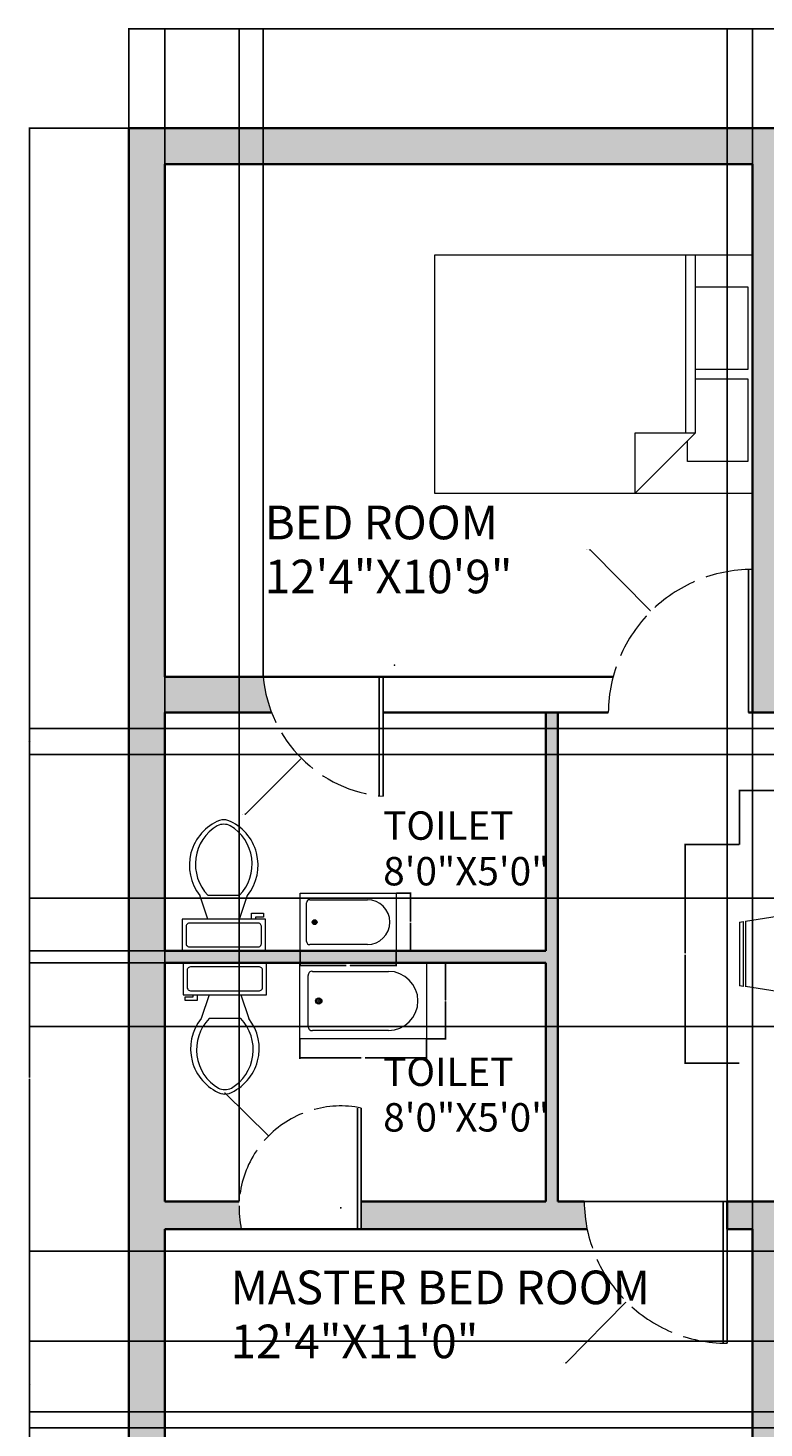
# Model space of a CAD drawing. Units: inches. Extents: x -12 to 539, y -477 to 51.
# Tile 2 of 6: x -12 to 173, y -301 to 51. Entities that reach past the tile are written whole.
import ezdxf

# ---------------------------------------------------------------- set-up
doc = ezdxf.new("R2010")
doc.units = ezdxf.units.IN
doc.header["$MEASUREMENT"] = 0
doc.linetypes.add('ACAD_ISO02W100', pattern=[15, 12, -3])
for name, color, linetype, lineweight in [('A-ANNO-DIMS', 2, 'Continuous', 18), ('A-AREA-IDEN', 7, 'Continuous', 18), ('A-DOOR', 4, 'Continuous', 25), ('A-DOOR-SWNG', 4, 'ACAD_ISO02W100', 13), ('A-FLOR-FIXT', 9, 'Continuous', 18), ('A-FURN', 8, 'Continuous', 18), ('A-WALL', 7, 'Continuous', 35)]:
    doc.layers.add(name, color=color, linetype=linetype, lineweight=lineweight)
doc.layers.add('A-WALL-PATT', color=252, linetype='Continuous', lineweight=13, true_color=0x939598)
doc.styles.get("Standard").update_dxf_attribs({"font": 'arial.ttf'})
doc.dimstyles.get("Standard").update_dxf_attribs({"dimtxt": 0.18, "dimasz": 0.18, "dimexe": 0.18, "dimexo": 0.0625, "dimgap": 0.09, "dimtad": 0, "dimtih": 1, "dimtoh": 1, "dimdec": 0, "dimzin": 0, "dimdsep": 46, "dimlunit": 3, "dimtxsty": 'Standard', "dimcen": 0.09, "dimadec": 0, "dimazin": 0, "dimtfac": 1, "dimtdec": 0, "dimtofl": 0, "dimtmove": 0, "dimatfit": 3, "dimfxl": 1, "dimtolj": 1, "dimtzin": 0, "dimarcsym": 0})

# ---------------------------------------------------------------- blocks, each defined once
blk = doc.blocks.new('Toilet - top')
for p, q in [((9.5, -6), (9.5, -2)), ((-10, -8.5), (-8, -8.5)), ((-10, -9.5), (-10, -8.5)), ((-7, -9.5), (-10, -9.5)), ((-8, -8.5), (-8, -8)), ((-7, -8), (-7, -9.5)), ((-4, -8), (-6, -14)), ((4, -8), (6, -14)), ((4, -14), (-4, -14))]:
    blk.add_line(p, q)
blk.add_lwpolyline([(10.5, -8), (10.5, 0), (-10.5, 0), (-10.5, -8)], close=True)
for points in [[(-9.5, -2), (-9.5, -6)], [(8.5, -1), (-8.5, -1)], [(-8.5, -7), (8.5, -7)]]:
    blk.add_lwpolyline(points)
for centre, radius, start, end in [((-8.62, -1.88), 0.884, 81.8699, 188.1301), ((8.62, -1.88), 0.884, 351.8699, 98.1301), ((-8.62, -6.12), 0.884, 171.8699, 278.1301), ((8.62, -6.12), 0.884, 261.8699, 8.1301), ((3.52, -21.58), 12.17, 141.4691, 247.9714), ((4.2, -21.82), 11.33, 136.3677, 238.9468), ((-3.52, -21.58), 12.17, 292.0284, 38.5307), ((-4.2, -21.82), 11.33, 301.053, 43.6321), ((0, -27.88), 4, 245.7318, 294.2682), ((0, -29), 4, 254.8605, 285.1395)]:
    blk.add_arc(centre, radius, start, end)
blk = doc.blocks.new('Bath Tub - 26 x 60 in.')
for p, q in [((8, -18), (10, -18)), ((9, -17), (9, -19))]:
    blk.add_line(p, q)
blk.add_lwpolyline([(0, -36), (0, 0), (60, 0), (60, -36)], close=True)
for points in [[(4, -30), (4, -6)], [(6, -4), (42, -4)], [(42, -32), (6, -32)]]:
    blk.add_lwpolyline(points)
for radius in [1.5, 1]:
    blk.add_circle((9, -18), radius)
for centre, radius, start, end in [((5.75, -5.75), 1.77, 81.8699, 188.1301), ((42, -18), 14, 270, 90), ((5.75, -30.25), 1.77, 171.8699, 278.1301)]:
    blk.add_arc(centre, radius, start, end)
blk = doc.blocks.new('Bed - Queen')
for p, q in [((0, -80.00003), (0, 0)), ((0, 0), (59.99999, 0)), ((59.99999, 0), (59.99999, -80.00003)), ((7.99999, -1.2), (28.79998, -1.2)), ((7.99999, -14.4), (7.99999, -1.2)), ((28.79998, -1.2), (28.79998, -14.4)), ((31.19999, -1.2), (51.99999, -1.2)), ((31.19999, -14.4), (31.19999, -1.2)), ((51.99999, -1.2), (51.99999, -16.4)), ((0, -14.4), (44.8, -14.4)), ((44.8, -16.8), (0, -16.8)), ((59.99999, -29.6), (44.8, -14.4)), ((44.8, -14.4), (44.8, -29.6)), ((51.99999, -16.4), (46.79936, -16.4)), ((44.8, -29.6), (59.99999, -29.6)), ((59.99999, -80.00003), (0, -80.00003))]:
    blk.add_line(p, q)
blk = doc.blocks.new('Dining Set - 36 x 72 in.')
for p, q in [((-22.2343, 26.00059), (-23.4847, 17.99762)), ((-22.2304, 26), (-5.7608, 26)), ((-22, 27.5), (-22.1562, 26.50042)), ((-5.8416, 26.5), (-22.1534, 26.5)), ((-22, 27.5), (-6, 27.5)), ((-5.8437, 26.49966), (-6, 27.5)), ((-4.5152, 17.99762), (-5.7655, 25.99926)), ((5.7657, 26.00059), (4.5153, 17.99762)), ((5.7696, 26), (22.2392, 26)), ((6, 27.5), (5.8438, 26.50042)), ((22.1584, 26.5), (5.8466, 26.5)), ((6, 27.5), (22, 27.5)), ((22.1563, 26.49966), (22, 27.5)), ((23.4848, 17.99762), (22.2345, 25.99926)), ((36, 18), (-36, 18)), ((-36, 18), (-36, -18)), ((36, -18), (36, 18)), ((-45.5, 8), (-44.5004, 8.15617)), ((-45.5, 8), (-45.5, -8)), ((-44.5, -8.15843), (-44.5, 8.15338)), ((-44.0006, 8.23428), (-35.9976, 9.48474)), ((-44, 8.23041), (-44, -8.23915)), ((44.0006, 8.23428), (35.9976, 9.48474)), ((44, 8.23041), (44, -8.23915)), ((44.5, -8.15843), (44.5, 8.15338)), ((45.5, 8), (44.5005, 8.15617)), ((45.5, 8), (45.5, -8)), ((-44.4997, -8.15631), (-45.5, -8)), ((-35.9976, -9.48476), (-43.9993, -8.2345)), ((35.9976, -9.48476), (43.9993, -8.2345)), ((44.4997, -8.15631), (45.5, -8)), ((-36, -18), (36, -18)), ((-22.2343, -26.0006), (-23.4847, -17.99762)), ((-4.5152, -17.99762), (-5.7655, -25.99928)), ((5.7657, -26.0006), (4.5153, -17.99762)), ((23.4848, -17.99762), (22.2345, -25.99928)), ((-22.2304, -26), (-5.7608, -26)), ((-22, -27.5), (-22.1562, -26.50044)), ((-5.8416, -26.5), (-22.1534, -26.5)), ((-22, -27.5), (-6, -27.5)), ((-5.8437, -26.49967), (-6, -27.5)), ((5.7696, -26), (22.2392, -26)), ((6, -27.5), (5.8438, -26.50044)), ((22.1584, -26.5), (5.8466, -26.5)), ((6, -27.5), (22, -27.5)), ((22.1563, -26.49967), (22, -27.5))]:
    blk.add_line(p, q)
for points in [[(-36, 15), (-31.1772, 14.97754), (-26.8079, 14.91406), (-22.8538, 14.81543), (-19.276, 14.6875), (-16.0362, 14.53613), (-13.0957, 14.36718), (-10.4159, 14.18652), (-7.9583, 14), (-5.6904, 13.81315), (-3.6035, 13.63021), (-1.6954, 13.45508), (0.0365, 13.29166), (1.5945, 13.14388), (2.9811, 13.01562), (4.1988, 12.9108), (5.25, 12.83333), (6.1393, 12.78613), (6.8802, 12.76823), (7.4883, 12.77767), (7.9792, 12.8125), (8.3685, 12.87077), (8.6719, 12.95052), (8.9049, 13.0498), (9.0833, 13.16666), (9.2205, 13.29899), (9.3216, 13.44401), (9.3895, 13.59879), (9.4271, 13.76041), (9.4373, 13.92594), (9.4232, 14.09245), (9.3875, 14.257), (9.3333, 14.41666), (9.2638, 14.56917), (9.1836, 14.71484), (9.0975, 14.85465), (9.0104, 14.98958), (8.9272, 15.1206), (8.8529, 15.2487), (8.7922, 15.37483), (8.75, 15.5), (8.7305, 15.62467), (8.7344, 15.74739), (8.7617, 15.86621), (8.8125, 15.97916), (8.8867, 16.08431), (8.9844, 16.17968), (9.1055, 16.26334), (9.25, 16.33333), (9.4189, 16.38802), (9.6172, 16.42708), (9.8506, 16.45052), (10.125, 16.45833), (10.4463, 16.45052), (10.8203, 16.42708), (11.2529, 16.38802), (11.75, 16.33333), (12.3184, 16.26318), (12.9694, 16.17838), (13.7151, 16.07991), (14.5677, 15.96875), (15.5395, 15.84586), (16.6426, 15.71224), (17.8893, 15.56884), (19.2917, 15.41666), (20.859, 15.25667), (22.5879, 15.08984), (24.4721, 14.91715), (26.5052, 14.73958), (28.6809, 14.5581), (30.9929, 14.3737), (33.4347, 14.18733), (36, 14)], [(-36, 10), (-28.9766, 10.14274), (-23.1725, 10.20442), (-18.4241, 10.19775), (-14.5677, 10.13541), (-11.4399, 10.03011), (-8.877, 9.89453), (-6.7154, 9.74137), (-4.7917, 9.58333), (-2.9698, 9.43082), (-1.2246, 9.28515), (0.4415, 9.14534), (2.026, 9.01041), (3.5266, 8.87939), (4.9408, 8.7513), (6.266, 8.62516), (7.5, 8.5), (8.6411, 8.37549), (9.6914, 8.2539), (10.6538, 8.13818), (11.5312, 8.03125), (12.3267, 7.93603), (13.043, 7.85547), (13.6831, 7.79248), (14.25, 7.75), (14.7471, 7.7303), (15.1797, 7.73307), (15.5537, 7.75732), (15.875, 7.80208), (16.1494, 7.86637), (16.3828, 7.94922), (16.5811, 8.04964), (16.75, 8.16666), (16.8944, 8.29915), (17.0143, 8.44531), (17.1089, 8.60319), (17.1771, 8.77083), (17.218, 8.94629), (17.2305, 9.1276), (17.2137, 9.31282), (17.1667, 9.5), (17.0895, 9.6875), (16.987, 9.875), (16.8649, 10.0625), (16.7292, 10.25), (16.5856, 10.4375), (16.4401, 10.625), (16.2985, 10.8125), (16.1667, 11), (16.05, 11.18733), (15.9518, 11.3737), (15.8752, 11.5581), (15.8229, 11.73958), (15.798, 11.91715), (15.8034, 12.08984), (15.842, 12.25667), (15.9167, 12.41666), (16.0295, 12.56836), (16.1784, 12.70833), (16.3605, 12.83268), (16.5729, 12.9375), (16.8127, 13.01888), (17.0768, 13.07291), (17.3625, 13.0957), (17.6667, 13.08333), (17.9894, 13.03312), (18.3418, 12.94726), (18.7382, 12.82918), (19.1927, 12.68229), (19.7195, 12.51001), (20.3327, 12.31575), (21.0465, 12.10294), (21.875, 11.875), (22.8357, 11.63354), (23.959, 11.37304), (25.2786, 11.08618), (26.8282, 10.76562), (28.6414, 10.40405), (30.752, 9.99414), (33.1936, 9.52856), (36, 9)], [(-36, 5.5), (-30.7157, 5.3348), (-26.069, 5.20963), (-21.9946, 5.11767), (-18.4271, 5.05208), (-15.3009, 5.00602), (-12.5508, 4.97265), (-10.1112, 4.94515), (-7.9167, 4.91666), (-5.909, 4.88167), (-4.0586, 4.83984), (-2.3429, 4.79215), (-0.7396, 4.73958), (0.7739, 4.6831), (2.22, 4.6237), (3.6213, 4.56233), (5, 4.5), (6.373, 4.43782), (7.7344, 4.3776), (9.0723, 4.32129), (10.375, 4.27083), (11.6309, 4.22819), (12.8281, 4.19531), (13.9551, 4.17415), (15, 4.16666), (15.954, 4.17448), (16.819, 4.19791), (17.6001, 4.23698), (18.3021, 4.29166), (18.9299, 4.36198), (19.4883, 4.44791), (19.9823, 4.54948), (20.4167, 4.66666), (20.7969, 4.79899), (21.1302, 4.94401), (21.4245, 5.09879), (21.6875, 5.26041), (21.9271, 5.42594), (22.1511, 5.59245), (22.3672, 5.757), (22.5834, 5.91666), (22.8065, 6.06868), (23.0404, 6.21093), (23.2879, 6.34147), (23.5521, 6.45833), (23.8358, 6.55957), (24.142, 6.64323), (24.4735, 6.70735), (24.8334, 6.75), (25.2235, 6.76969), (25.642, 6.76692), (26.0858, 6.74267), (26.5521, 6.69791), (27.0379, 6.63362), (27.5404, 6.55078), (28.0565, 6.45036), (28.5834, 6.33333), (29.1242, 6.19987), (29.7071, 6.04687), (30.3661, 5.87044), (31.1354, 5.66666), (32.0493, 5.43164), (33.142, 5.16146), (34.4475, 4.85221), (36, 4.5)], [(-36, -1), (-30.7915, -0.6591), (-26.0195, -0.38216), (-21.6519, -0.16284), (-17.6563, 0.00521), (-14.0005, 0.12833), (-10.6523, 0.21289), (-7.5796, 0.26522), (-4.75, 0.29166), (-2.134, 0.29793), (0.2878, 0.28711), (2.5317, 0.26163), (4.6146, 0.22396), (6.5529, 0.17651), (8.3633, 0.12174), (10.0623, 0.06209), (11.6667, 0), (13.1899, -0.06201), (14.6341, -0.1211), (15.9982, -0.17432), (17.2813, -0.21875), (18.4823, -0.25147), (19.6003, -0.26953), (20.6343, -0.27002), (21.5834, -0.25), (22.4481, -0.20768), (23.2357, -0.14584), (23.9549, -0.06836), (24.6146, 0.02083), (25.2235, 0.11784), (25.7904, 0.21875), (26.3241, 0.31966), (26.8334, 0.41666), (27.3265, 0.50618), (27.8099, 0.58593), (28.2894, 0.65397), (28.7709, 0.70833), (29.2601, 0.74707), (29.763, 0.76823), (30.2855, 0.76985), (30.8334, 0.75), (31.4088, 0.70784), (31.9994, 0.64713), (32.589, 0.57275), (33.1615, 0.48958), (33.7008, 0.4025), (34.1908, 0.3164), (34.6153, 0.23616), (34.9584, 0.16666), (35.2099, 0.11165), (35.3848, 0.07031), (35.504, 0.04069), (35.5886, 0.02083), (35.6594, 0.00879), (35.7377, 0.0026), (35.8442, 0.00032), (36, 0)], [(-36, -6.5), (-27.1843, -6.31267), (-20.084, -6.1263), (-14.469, -5.9419), (-10.1094, -5.76042), (-6.7752, -5.58285), (-4.2363, -5.41016), (-2.2629, -5.24333), (-0.625, -5.08334), (0.8708, -4.93099), (2.2715, -4.78646), (3.5872, -4.64974), (4.8281, -4.52084), (6.0046, -4.39974), (7.127, -4.28646), (8.2053, -4.18099), (9.25, -4.08334), (10.2705, -3.99382), (11.2734, -3.91407), (12.2647, -3.84603), (13.25, -3.79167), (14.2354, -3.75293), (15.2266, -3.73177), (16.2295, -3.73015), (17.25, -3.75), (18.2912, -3.79248), (19.3451, -3.85547), (20.4009, -3.93604), (21.4479, -4.03125), (22.4754, -4.13819), (23.4727, -4.25391), (24.4289, -4.37549), (25.3334, -4.5), (26.1785, -4.62492), (26.9694, -4.74935), (27.7145, -4.87281), (28.4219, -4.99479), (29.1, -5.11483), (29.7572, -5.23242), (30.4016, -5.34709), (31.0417, -5.45834), (31.6837, -5.56437), (32.3262, -5.65821), (32.9658, -5.73153), (33.599, -5.77604), (34.2224, -5.78345), (34.8327, -5.74545), (35.4264, -5.65373), (36, -5.5)], [(-36, -10), (-26.4022, -9.81299), (-18.4675, -9.62891), (-11.9839, -9.45069), (-6.7396, -9.28125), (-2.5226, -9.12354), (0.8789, -8.98047), (3.6769, -8.85498), (6.0833, -8.75), (8.2767, -8.66765), (10.3021, -8.60677), (12.1712, -8.56543), (13.8958, -8.54167), (15.4876, -8.53353), (16.9583, -8.53907), (18.3197, -8.55632), (19.5834, -8.58334), (20.7616, -8.61841), (21.8685, -8.66081), (22.9188, -8.71004), (23.9271, -8.76563), (24.9081, -8.82707), (25.8763, -8.89388), (26.8465, -8.96558), (27.8334, -9.04167), (28.8474, -9.12118), (29.8828, -9.20117), (30.93, -9.27824), (31.9792, -9.34896), (33.0205, -9.40991), (34.0443, -9.45768), (35.0407, -9.48885), (36, -9.5)], [(-36, -14.5), (-30.0881, -14.33513), (-25.0332, -14.21224), (-20.7312, -14.12647), (-17.0781, -14.07292), (-13.97, -14.04671), (-11.3027, -14.04297), (-8.9724, -14.05681), (-6.875, -14.08334), (-4.9224, -14.11833), (-3.0905, -14.16016), (-1.3709, -14.20785), (0.2448, -14.26042), (1.7647, -14.3169), (3.1973, -14.3763), (4.5507, -14.43767), (5.8333, -14.5), (7.0554, -14.5621), (8.235, -14.62175), (9.3922, -14.67652), (10.5469, -14.72396), (11.7192, -14.76164), (12.929, -14.78711), (14.1965, -14.79794), (15.5417, -14.79167), (16.9933, -14.76424), (18.6152, -14.70508), (20.4804, -14.60197), (22.6615, -14.44271), (25.2312, -14.21509), (28.2624, -13.9069), (31.8277, -13.50594), (36, -13)]]:
    blk.add_lwpolyline(points)
blk = doc.blocks.new('*D19')
at = {"layer": 'A-ANNO-DIMS', "color": 0, "lineweight": -2, "transparency": 16777216}
for p, q in [((56.22, -181.05), (56.22, -184.79)), ((80.4, -181.05), (80.4, -184.79)), ((56.4, -184.61), (67.8, -184.61)), ((80.22, -184.61), (68.82, -184.61))]:
    blk.add_line(p, q, dxfattribs=at)
at = {"layer": 'A-ANNO-DIMS', "color": 0, "transparency": 16777216}
for points in [[(56.4, -184.58), (56.4, -184.64), (56.22, -184.61)], [(80.22, -184.58), (80.22, -184.64), (80.4, -184.61)]]:
    blk.add_solid(points, dxfattribs=at)
at = {"layer": 'Defpoints', "color": 0, "transparency": 16777216}
for p in [(56.22, -180.99), (80.4, -180.99), (80.4, -184.61)]:
    blk.add_point(p, dxfattribs=at)
at = {"layer": 'A-ANNO-DIMS', "color": 0, "transparency": 16777216, "insert": (68.31, -184.61), "char_height": 0.18, "attachment_point": 5}
blk.add_mtext('\\A1;TUB 24', dxfattribs=at)
blk = doc.blocks.new('*D20')
at = {"layer": 'A-ANNO-DIMS', "color": 0, "lineweight": -2, "transparency": 16777216}
for p, q in [((80.46, -166.48), (84.2, -166.48)), ((84.02, -166.66), (84.02, -173.55)), ((84.02, -180.81), (84.02, -173.92)), ((80.46, -180.99), (84.2, -180.99))]:
    blk.add_line(p, q, dxfattribs=at)
at = {"layer": 'A-ANNO-DIMS', "color": 0, "transparency": 16777216}
for points in [[(83.99, -166.66), (84.05, -166.66), (84.02, -166.48)], [(83.99, -180.81), (84.05, -180.81), (84.02, -180.99)]]:
    blk.add_solid(points, dxfattribs=at)
at = {"layer": 'Defpoints', "color": 0, "transparency": 16777216}
for p in [(80.4, -166.48), (84.02, -166.48), (80.4, -180.99)]:
    blk.add_point(p, dxfattribs=at)
at = {"layer": 'A-ANNO-DIMS', "color": 0, "transparency": 16777216, "insert": (84.02, -173.73), "char_height": 0.18, "attachment_point": 5}
blk.add_mtext('\\A1;15', dxfattribs=at)
blk = doc.blocks.new('*D21')
at = {"layer": 'A-ANNO-DIMS', "color": 0, "lineweight": -2, "transparency": 16777216}
for p, q in [((56.1, -203.19), (56.1, -208.09)), ((88, -203.19), (88, -208.09)), ((56.28, -207.91), (71.54, -207.91)), ((87.82, -207.91), (72.56, -207.91))]:
    blk.add_line(p, q, dxfattribs=at)
at = {"layer": 'A-ANNO-DIMS', "color": 0, "transparency": 16777216}
for points in [[(56.28, -207.88), (56.28, -207.94), (56.1, -207.91)], [(87.82, -207.88), (87.82, -207.94), (88, -207.91)]]:
    blk.add_solid(points, dxfattribs=at)
at = {"layer": 'Defpoints', "color": 0, "transparency": 16777216}
for p in [(56.1, -203.12), (88, -203.12), (88, -207.91)]:
    blk.add_point(p, dxfattribs=at)
at = {"layer": 'A-ANNO-DIMS', "color": 0, "transparency": 16777216, "insert": (72.05, -207.91), "char_height": 0.18, "attachment_point": 5}
blk.add_mtext('\\A1;TUB 32', dxfattribs=at)
blk = doc.blocks.new('*D22')
at = {"layer": 'A-ANNO-DIMS', "color": 0, "lineweight": -2, "transparency": 16777216}
for p, q in [((88.06, -183.99), (92.96, -183.99)), ((92.78, -184.17), (92.78, -193.37)), ((92.78, -202.94), (92.78, -193.74)), ((88.06, -203.12), (92.96, -203.12))]:
    blk.add_line(p, q, dxfattribs=at)
at = {"layer": 'A-ANNO-DIMS', "color": 0, "transparency": 16777216}
for points in [[(92.75, -184.17), (92.81, -184.17), (92.78, -183.99)], [(92.75, -202.94), (92.81, -202.94), (92.78, -203.12)]]:
    blk.add_solid(points, dxfattribs=at)
at = {"layer": 'Defpoints', "color": 0, "transparency": 16777216}
for p in [(88, -183.99), (92.78, -183.99), (88, -203.12)]:
    blk.add_point(p, dxfattribs=at)
at = {"layer": 'A-ANNO-DIMS', "color": 0, "transparency": 16777216, "insert": (92.78, -193.56), "char_height": 0.18, "attachment_point": 5}
blk.add_mtext('\\A1;19', dxfattribs=at)
blk = doc.blocks.new('*D29')
at = {"layer": 'A-ANNO-DIMS', "color": 0, "lineweight": -2, "transparency": 16777216}
for p, q in [((166.81, -154.17), (166.81, -140.4)), ((166.99, -140.58), (211.36, -140.58)), ((257.63, -140.58), (213.27, -140.58)), ((257.81, -154.17), (257.81, -140.4))]:
    blk.add_line(p, q, dxfattribs=at)
at = {"layer": 'A-ANNO-DIMS', "color": 0, "transparency": 16777216}
for points in [[(166.99, -140.55), (166.99, -140.61), (166.81, -140.58)], [(257.63, -140.55), (257.63, -140.61), (257.81, -140.58)]]:
    blk.add_solid(points, dxfattribs=at)
at = {"layer": 'Defpoints', "color": 0, "transparency": 16777216}
for p in [(257.81, -140.58), (166.81, -154.23), (257.81, -154.23)]:
    blk.add_point(p, dxfattribs=at)
at = {"layer": 'A-ANNO-DIMS', "color": 0, "transparency": 16777216, "insert": (212.31, -140.58), "char_height": 0.18, "attachment_point": 5}
blk.add_mtext('\\A1;DINING SET 91', dxfattribs=at)
blk = doc.blocks.new('*D30')
at = {"layer": 'A-ANNO-DIMS', "color": 0, "lineweight": -2, "transparency": 16777216}
for p, q in [((166.75, -154.23), (152.98, -154.23)), ((153.16, -154.41), (153.16, -181.55)), ((153.16, -209.05), (153.16, -181.92)), ((166.75, -209.23), (152.98, -209.23))]:
    blk.add_line(p, q, dxfattribs=at)
at = {"layer": 'A-ANNO-DIMS', "color": 0, "transparency": 16777216}
for points in [[(153.13, -154.41), (153.19, -154.41), (153.16, -154.23)], [(153.13, -209.05), (153.19, -209.05), (153.16, -209.23)]]:
    blk.add_solid(points, dxfattribs=at)
at = {"layer": 'Defpoints', "color": 0, "transparency": 16777216}
for p in [(153.16, -154.23), (166.81, -154.23), (166.81, -209.23)]:
    blk.add_point(p, dxfattribs=at)
at = {"layer": 'A-ANNO-DIMS', "color": 0, "transparency": 16777216, "insert": (153.16, -181.73), "char_height": 0.18, "attachment_point": 5}
blk.add_mtext('\\A1;55', dxfattribs=at)
blk = doc.blocks.new('*D37')
at = {"layer": 'A-ANNO-DIMS', "color": 0, "lineweight": -2, "transparency": 16777216}
for p, q in [((13.1, 26.07), (13.1, 51.25)), ((13.28, 51.07), (263.15, 51.07)), ((513.81, 51.07), (263.94, 51.07)), ((513.99, -124.93), (513.99, 51.25))]:
    blk.add_line(p, q, dxfattribs=at)
at = {"layer": 'A-ANNO-DIMS', "color": 0, "transparency": 16777216}
for points in [[(13.28, 51.1), (13.28, 51.04), (13.1, 51.07)], [(513.81, 51.1), (513.81, 51.04), (513.99, 51.07)]]:
    blk.add_solid(points, dxfattribs=at)
at = {"layer": 'Defpoints', "color": 0, "transparency": 16777216}
for p in [(513.99, 51.07), (13.1, 26.01), (513.99, -124.99)]:
    blk.add_point(p, dxfattribs=at)
at = {"layer": 'A-ANNO-DIMS', "color": 0, "transparency": 16777216, "insert": (263.54, 51.07), "char_height": 0.18, "attachment_point": 5}
blk.add_mtext('\\A1;500.9', dxfattribs=at)
blk = doc.blocks.new('*D38')
at = {"layer": 'A-ANNO-DIMS', "color": 0, "lineweight": -2, "transparency": 16777216}
for p, q in [((13.04, 26.01), (-12.14, 26.01)), ((-11.96, 25.83), (-11.96, -212.81)), ((-11.96, -451.81), (-11.96, -213.17)), ((168.04, -451.99), (-12.14, -451.99))]:
    blk.add_line(p, q, dxfattribs=at)
at = {"layer": 'A-ANNO-DIMS', "color": 0, "transparency": 16777216}
for points in [[(-11.99, 25.83), (-11.93, 25.83), (-11.96, 26.01)], [(-11.99, -451.81), (-11.93, -451.81), (-11.96, -451.99)]]:
    blk.add_solid(points, dxfattribs=at)
at = {"layer": 'Defpoints', "color": 0, "transparency": 16777216}
for p in [(13.1, 26.01), (-11.96, -451.99), (168.1, -451.99)]:
    blk.add_point(p, dxfattribs=at)
at = {"layer": 'A-ANNO-DIMS', "color": 0, "transparency": 16777216, "insert": (-11.96, -212.99), "char_height": 0.18, "attachment_point": 5}
blk.add_mtext('\\A1;478', dxfattribs=at)
blk = doc.blocks.new('*D46')
at = {"layer": 'A-ANNO-DIMS', "color": 0, "lineweight": -2, "transparency": 16777216}
for p, q in [((170.1, 17.07), (170.1, 51.25)), ((170.28, 51.07), (173.45, 51.07)), ((176.92, 51.07), (173.75, 51.07)), ((177.1, 17.07), (177.1, 51.25))]:
    blk.add_line(p, q, dxfattribs=at)
at = {"layer": 'A-ANNO-DIMS', "color": 0, "transparency": 16777216}
for points in [[(170.28, 51.1), (170.28, 51.04), (170.1, 51.07)], [(176.92, 51.1), (176.92, 51.04), (177.1, 51.07)]]:
    blk.add_solid(points, dxfattribs=at)
at = {"layer": 'Defpoints', "color": 0, "transparency": 16777216}
for p in [(177.1, 51.07), (170.1, 17.01), (177.1, 17.01)]:
    blk.add_point(p, dxfattribs=at)
at = {"layer": 'A-ANNO-DIMS', "color": 0, "transparency": 16777216, "insert": (173.6, 51.07), "char_height": 0.18, "attachment_point": 5}
blk.add_mtext('\\A1;7', dxfattribs=at)
blk = doc.blocks.new('*D47')
at = {"layer": 'A-ANNO-DIMS', "color": 0, "lineweight": -2, "transparency": 16777216}
for p, q in [((22.04, -180.99), (-12.14, -180.99)), ((-11.96, -181.17), (-11.96, -182.31)), ((-11.96, -183.81), (-11.96, -182.67)), ((22.04, -183.99), (-12.14, -183.99))]:
    blk.add_line(p, q, dxfattribs=at)
at = {"layer": 'A-ANNO-DIMS', "color": 0, "transparency": 16777216}
for points in [[(-11.99, -181.17), (-11.93, -181.17), (-11.96, -180.99)], [(-11.99, -183.81), (-11.93, -183.81), (-11.96, -183.99)]]:
    blk.add_solid(points, dxfattribs=at)
at = {"layer": 'Defpoints', "color": 0, "transparency": 16777216}
for p in [(22.1, -180.99), (-11.96, -183.99), (22.1, -183.99)]:
    blk.add_point(p, dxfattribs=at)
at = {"layer": 'A-ANNO-DIMS', "color": 0, "transparency": 16777216, "insert": (-11.96, -182.49), "char_height": 0.18, "attachment_point": 5}
blk.add_mtext('\\A1;3', dxfattribs=at)
blk = doc.blocks.new('*D48')
at = {"layer": 'A-ANNO-DIMS', "color": 0, "lineweight": -2, "transparency": 16777216}
for p, q in [((22.1, -111.93), (22.1, 51.25)), ((22.28, 51.07), (34.04, 51.07)), ((46.73, 51.07), (34.97, 51.07)), ((46.91, -111.93), (46.91, 51.25))]:
    blk.add_line(p, q, dxfattribs=at)
at = {"layer": 'A-ANNO-DIMS', "color": 0, "transparency": 16777216}
for points in [[(22.28, 51.1), (22.28, 51.04), (22.1, 51.07)], [(46.73, 51.1), (46.73, 51.04), (46.91, 51.07)]]:
    blk.add_solid(points, dxfattribs=at)
at = {"layer": 'Defpoints', "color": 0, "transparency": 16777216}
for p in [(46.91, 51.07), (22.1, -111.99), (46.91, -111.99)]:
    blk.add_point(p, dxfattribs=at)
at = {"layer": 'A-ANNO-DIMS', "color": 0, "transparency": 16777216, "insert": (34.51, 51.07), "char_height": 0.18, "attachment_point": 5}
blk.add_mtext('\\A1;24.805', dxfattribs=at)
blk = doc.blocks.new('*D49')
at = {"layer": 'A-ANNO-DIMS', "color": 0, "lineweight": -2, "transparency": 16777216}
for p, q in [((22.1, -243.93), (22.1, 51.25)), ((22.28, 51.07), (31.1, 51.07)), ((40.68, 51.07), (31.87, 51.07)), ((40.86, -243.93), (40.86, 51.25))]:
    blk.add_line(p, q, dxfattribs=at)
at = {"layer": 'A-ANNO-DIMS', "color": 0, "transparency": 16777216}
for points in [[(22.28, 51.1), (22.28, 51.04), (22.1, 51.07)], [(40.68, 51.1), (40.68, 51.04), (40.86, 51.07)]]:
    blk.add_solid(points, dxfattribs=at)
at = {"layer": 'Defpoints', "color": 0, "transparency": 16777216}
for p in [(40.86, 51.07), (22.1, -243.99), (40.86, -243.99)]:
    blk.add_point(p, dxfattribs=at)
at = {"layer": 'A-ANNO-DIMS', "color": 0, "transparency": 16777216, "insert": (31.48, 51.07), "char_height": 0.18, "attachment_point": 5}
blk.add_mtext('\\A1;18.76', dxfattribs=at)
blk = doc.blocks.new('*D50')
at = {"layer": 'A-ANNO-DIMS', "color": 0, "lineweight": -2, "transparency": 16777216}
for p, q in [((321.04, -167.71), (-12.14, -167.71)), ((-11.96, -167.89), (-11.96, -183.67)), ((-11.96, -199.81), (-11.96, -184.03)), ((328.04, -199.99), (-12.14, -199.99))]:
    blk.add_line(p, q, dxfattribs=at)
at = {"layer": 'A-ANNO-DIMS', "color": 0, "transparency": 16777216}
for points in [[(-11.99, -167.89), (-11.93, -167.89), (-11.96, -167.71)], [(-11.99, -199.81), (-11.93, -199.81), (-11.96, -199.99)]]:
    blk.add_solid(points, dxfattribs=at)
at = {"layer": 'Defpoints', "color": 0, "transparency": 16777216}
for p in [(-11.96, -167.71), (321.1, -167.71), (328.1, -199.99)]:
    blk.add_point(p, dxfattribs=at)
at = {"layer": 'A-ANNO-DIMS', "color": 0, "transparency": 16777216, "insert": (-11.96, -183.85), "char_height": 0.18, "attachment_point": 5}
blk.add_mtext('\\A1;32.274', dxfattribs=at)
blk = doc.blocks.new('*D53')
at = {"layer": 'A-ANNO-DIMS', "color": 0, "lineweight": -2, "transparency": 16777216}
for p, q in [((379.04, -124.99), (-12.14, -124.99)), ((-11.96, -125.17), (-11.96, -128.09)), ((-11.96, -131.38), (-11.96, -128.46)), ((379.04, -131.56), (-12.14, -131.56))]:
    blk.add_line(p, q, dxfattribs=at)
at = {"layer": 'A-ANNO-DIMS', "color": 0, "transparency": 16777216}
for points in [[(-11.99, -125.17), (-11.93, -125.17), (-11.96, -124.99)], [(-11.99, -131.38), (-11.93, -131.38), (-11.96, -131.56)]]:
    blk.add_solid(points, dxfattribs=at)
at = {"layer": 'Defpoints', "color": 0, "transparency": 16777216}
for p in [(379.1, -124.99), (-11.96, -131.56), (379.1, -131.56)]:
    blk.add_point(p, dxfattribs=at)
at = {"layer": 'A-ANNO-DIMS', "color": 0, "transparency": 16777216, "insert": (-11.96, -128.27), "char_height": 0.18, "attachment_point": 5}
blk.add_mtext('\\A1;6.575', dxfattribs=at)
blk = doc.blocks.new('*D54')
at = {"layer": 'A-ANNO-DIMS', "color": 0, "lineweight": -2, "transparency": 16777216}
for p, q in [((321.04, -256.55), (-12.14, -256.55)), ((-11.96, -256.73), (-11.96, -276.57)), ((-11.96, -296.78), (-11.96, -276.93)), ((321.04, -296.96), (-12.14, -296.96))]:
    blk.add_line(p, q, dxfattribs=at)
at = {"layer": 'A-ANNO-DIMS', "color": 0, "transparency": 16777216}
for points in [[(-11.99, -256.73), (-11.93, -256.73), (-11.96, -256.55)], [(-11.99, -296.78), (-11.93, -296.78), (-11.96, -296.96)]]:
    blk.add_solid(points, dxfattribs=at)
at = {"layer": 'Defpoints', "color": 0, "transparency": 16777216}
for p in [(321.1, -256.55), (-11.96, -296.96), (321.1, -296.96)]:
    blk.add_point(p, dxfattribs=at)
at = {"layer": 'A-ANNO-DIMS', "color": 0, "transparency": 16777216, "insert": (-11.96, -276.75), "char_height": 0.18, "attachment_point": 5}
blk.add_mtext('\\A1;40.41', dxfattribs=at)
blk = doc.blocks.new('*D57')
at = {"layer": 'A-ANNO-DIMS', "color": 0, "lineweight": -2, "transparency": 16777216}
for p, q in [((163.73, -250.93), (163.73, 51.25)), ((163.91, 51.07), (166.52, 51.07)), ((169.92, 51.07), (167.31, 51.07)), ((170.1, -250.93), (170.1, 51.25))]:
    blk.add_line(p, q, dxfattribs=at)
at = {"layer": 'A-ANNO-DIMS', "color": 0, "transparency": 16777216}
for points in [[(163.91, 51.1), (163.91, 51.04), (163.73, 51.07)], [(169.92, 51.1), (169.92, 51.04), (170.1, 51.07)]]:
    blk.add_solid(points, dxfattribs=at)
at = {"layer": 'Defpoints', "color": 0, "transparency": 16777216}
for p in [(163.73, 51.07), (163.73, -250.99), (170.1, -250.99)]:
    blk.add_point(p, dxfattribs=at)
at = {"layer": 'A-ANNO-DIMS', "color": 0, "transparency": 16777216, "insert": (166.92, 51.07), "char_height": 0.18, "attachment_point": 5}
blk.add_mtext('\\A1;6.372', dxfattribs=at)
blk = doc.blocks.new('*D60')
at = {"layer": 'A-ANNO-DIMS', "color": 0, "lineweight": -2, "transparency": 16777216}
for p, q in [((240.07, -279.21), (-12.14, -279.21)), ((-11.96, -279.39), (-11.96, -289.91)), ((-11.96, -300.79), (-11.96, -290.27)), ((240.07, -300.97), (-12.14, -300.97))]:
    blk.add_line(p, q, dxfattribs=at)
at = {"layer": 'A-ANNO-DIMS', "color": 0, "transparency": 16777216}
for points in [[(-11.99, -279.39), (-11.93, -279.39), (-11.96, -279.21)], [(-11.99, -300.79), (-11.93, -300.79), (-11.96, -300.97)]]:
    blk.add_solid(points, dxfattribs=at)
at = {"layer": 'Defpoints', "color": 0, "transparency": 16777216}
for p in [(240.14, -279.21), (-11.96, -300.97), (240.14, -300.97)]:
    blk.add_point(p, dxfattribs=at)
at = {"layer": 'A-ANNO-DIMS', "color": 0, "transparency": 16777216, "insert": (-11.96, -290.09), "char_height": 0.18, "attachment_point": 5}
blk.add_mtext('\\A1;21.76', dxfattribs=at)
blk = doc.blocks.new('*D61')
at = {"layer": 'A-ANNO-DIMS', "color": 0, "lineweight": -2, "transparency": 16777216}
for p, q in [((129.03, -80.05), (129.21, -80.05)), ((129.21, -80.05), (144.42, -95.39)), ((170.01, -121.28), (170.19, -121.28)), ((170.1, -121.37), (170.1, -121.19))]:
    blk.add_line(p, q, dxfattribs=at)
at = {"layer": 'A-ANNO-DIMS', "color": 0, "transparency": 16777216}
blk.add_solid([(144.44, -95.37), (144.39, -95.41), (144.54, -95.51)], dxfattribs=at)
at = {"layer": 'Defpoints', "color": 0, "transparency": 16777216}
for p in [(144.54, -95.51), (170.1, -121.28)]:
    blk.add_point(p, dxfattribs=at)
at = {"layer": 'A-ANNO-DIMS', "color": 0, "transparency": 16777216, "insert": (128.62, -80.05), "char_height": 0.18, "attachment_point": 5}
blk.add_mtext('\\A1;R36.3', dxfattribs=at)
blk = doc.blocks.new('*D64')
at = {"layer": 'A-ANNO-DIMS', "color": 0, "lineweight": -2, "transparency": 16777216}
for p, q in [((163.64, -243.69), (163.82, -243.69)), ((163.73, -243.78), (163.73, -243.6)), ((123.17, -284.59), (138.25, -269.38)), ((122.99, -284.59), (123.17, -284.59))]:
    blk.add_line(p, q, dxfattribs=at)
at = {"layer": 'A-ANNO-DIMS', "color": 0, "transparency": 16777216}
blk.add_solid([(138.23, -269.36), (138.27, -269.4), (138.38, -269.25)], dxfattribs=at)
at = {"layer": 'Defpoints', "color": 0, "transparency": 16777216}
for p in [(163.73, -243.69), (138.38, -269.25)]:
    blk.add_point(p, dxfattribs=at)
at = {"layer": 'A-ANNO-DIMS', "color": 0, "transparency": 16777216, "insert": (122.68, -284.59), "char_height": 0.18, "attachment_point": 5}
blk.add_mtext('\\A1;R36', dxfattribs=at)
blk = doc.blocks.new('*D66')
at = {"layer": 'A-ANNO-DIMS', "color": 0, "lineweight": -2, "transparency": 16777216}
for p, q in [((79.85, -109.04), (80.03, -109.04)), ((79.94, -109.13), (79.94, -108.95)), ((42.47, -146.6), (56.39, -132.64)), ((42.29, -146.6), (42.47, -146.6))]:
    blk.add_line(p, q, dxfattribs=at)
at = {"layer": 'A-ANNO-DIMS', "color": 0, "transparency": 16777216}
blk.add_solid([(56.37, -132.62), (56.41, -132.66), (56.52, -132.52)], dxfattribs=at)
at = {"layer": 'Defpoints', "color": 0, "transparency": 16777216}
for p in [(79.94, -109.04), (56.52, -132.52)]:
    blk.add_point(p, dxfattribs=at)
at = {"layer": 'A-ANNO-DIMS', "color": 0, "transparency": 16777216, "insert": (41.81, -146.6), "char_height": 0.18, "attachment_point": 5}
blk.add_mtext('\\A1;R33.16', dxfattribs=at)
blk = doc.blocks.new('*D68')
at = {"layer": 'A-ANNO-DIMS', "color": 0, "lineweight": -2, "transparency": 16777216}
for p, q in [((37.15, -216.75), (37.33, -216.75)), ((37.33, -216.75), (48.11, -227.44)), ((66.32, -245.59), (66.5, -245.59)), ((66.41, -245.68), (66.41, -245.5))]:
    blk.add_line(p, q, dxfattribs=at)
at = {"layer": 'A-ANNO-DIMS', "color": 0, "transparency": 16777216}
blk.add_solid([(48.13, -227.41), (48.09, -227.46), (48.23, -227.56)], dxfattribs=at)
at = {"layer": 'Defpoints', "color": 0, "transparency": 16777216}
for p in [(48.23, -227.56), (66.41, -245.59)]:
    blk.add_point(p, dxfattribs=at)
at = {"layer": 'A-ANNO-DIMS', "color": 0, "transparency": 16777216, "insert": (36.74, -216.75), "char_height": 0.18, "attachment_point": 5}
blk.add_mtext('\\A1;R25.6', dxfattribs=at)

msp = doc.modelspace()

# ---------------------------------------------------------------- hatches: boundary and pattern name
at = {"layer": 'A-WALL-PATT'}
h = msp.add_hatch(color=256, dxfattribs=at)
h.dxf.hatch_style = 1
h.paths.add_polyline_path([(267.143, 26.0124), (13.1031, 26.0124), (13.1031, -391.9876), (177.1031, -391.9876), (177.1031, -346.9876), (307.7315, -346.9876), (321.1031, -346.9876), (321.1031, -389.9876), (469.1031, -389.9876), (469.1031, 26.0124), (302.7142, 26.0124), (302.7142, 17.0124), (321.1031, 17.0124), (321.1031, -131.577, -0.04877504), (328.1031, -132.2621), (328.1031, 17.0124), (460.1031, 17.0124), (460.1031, -124.9876), (382.1031, -124.9876), (379.1031, -124.9876), (379.1031, -131.5624), (382.1031, -131.5624), (382.1031, -127.9876), (460.1031, -127.9876), (460.1031, -153.7747), (460.1031, -199.9876), (382.1031, -199.9876), (382.1031, -167.7132), (379.1031, -167.7132), (379.1031, -199.9876), (328.1031, -199.9876), (328.1031, -167.7132), (321.1031, -167.7132), (321.1031, -206.9876), (460.1031, -206.9876), (460.1031, -323.9876), (388.677, -323.9876, -0.02504709), (388.5266, -326.9876), (460.1031, -326.9876), (460.1031, -380.9876), (328.1031, -380.9876), (328.1031, -326.9876), (358.677, -326.9876), (358.677, -323.9876), (328.1031, -323.9876), (328.1031, -296.9562), (321.1031, -296.9562), (321.1031, -339.9876), (307.7315, -339.9876), (177.1031, -339.9876), (177.1031, -250.9876), (244.0259, -250.9876), (244.0259, -243.9876), (163.7315, -243.9876), (163.7315, -250.9876), (170.1031, -250.9876), (170.1031, -382.9876), (22.1031, -382.9876), (22.1031, -250.9876), (41.3871, -250.9876, -0.06888376), (40.8612, -243.9876), (22.1031, -243.9876), (22.1031, -183.9876), (118.1031, -183.9876), (118.1031, -243.9876), (71.6031, -243.9876), (71.6031, -250.9876), (128.4772, -250.9876, -0.04900189), (127.7315, -243.9876), (121.1031, -243.9876), (121.1031, -183.9876), (121.1031, -120.9876), (118.1031, -120.9876), (118.1031, -180.9876), (22.1031, -180.9876), (22.1031, -120.9876), (49.0045, -120.9876, -0.07000725), (46.9084, -111.9876), (46.1728, -111.9876), (22.1031, -111.9876), (22.1031, 17.0124), (170.1031, 17.0124), (170.1031, -120.9876), (177.1031, -120.9876), (177.1031, 17.0124), (268.2584, 17.0124, -0.0639977)])
h.paths.add_polyline_path([(513.9866, -124.9876), (469.1031, -124.9876), (469.1031, -127.9876), (510.9866, -127.9876), (510.9866, -259.2045), (469.1031, -259.2045), (469.1031, -262.2045), (513.9866, -262.2045)])
h.paths.add_polyline_path([(351.8833, -206.9876), (348.8833, -206.9876), (348.8833, -253.547), (328.1031, -253.547), (321.1031, -253.547), (321.1031, -256.547), (328.1031, -256.547), (351.8833, -256.547)], flags=17)
h.paths.add_polyline_path([(330.1031, -389.9876), (321.1031, -389.9876), (321.1031, -442.9876), (177.1031, -442.9876), (177.1031, -391.9876), (168.1031, -391.9876), (168.1031, -451.9876), (330.1031, -451.9876)])
h.paths.add_polyline_path([(414.1504, -177.6962), (465.5248, -177.6962), (465.5248, -164.7437), (414.1504, -164.7437)], flags=25)

# ---------------------------------------------------------------- linework, layer by layer
at = {"layer": 'A-DOOR'}
for p, q in [((169.1031, -120.9876), (169.1031, -84.9876)), ((170.1031, -120.9876), (170.1031, -84.9876)), ((77.068, -111.9876), (46.1728, -111.9876)), ((76.068, -111.9876), (76.068, -142.0759)), ((77.068, -111.9876), (77.068, -142.0759)), ((70.6031, -250.9876), (70.6031, -220.5228)), ((71.6031, -250.9876), (71.6031, -220.5228)), ((163.7315, -243.9876), (127.7315, -243.9876)), ((162.7315, -243.9876), (162.7315, -279.6935)), ((163.7315, -243.9876), (163.7315, -279.6935)), ((71.6031, -250.9876), (41.3871, -250.9876)), ((41.3871, -250.9876), (41.3871, -250.9876))]:
    msp.add_line(p, q, dxfattribs=at)
at = {"layer": 'A-DOOR-SWNG'}
for centre, radius, start, end in [((170.1031, -121.2845), 36.2969, 90, 179.531256), ((79.9385, -109.0389), 33.1614, 185.101364, 265.03415), ((66.4087, -245.5879), 25.5976, 78.2921, 192.177774), ((163.7315, -243.6923), 36.0012, 180.469881, 270)]:
    msp.add_arc(centre, radius, start, end, dxfattribs=at)
at = {"layer": 'A-WALL'}
for p, q in [((13.1031, 26.0124), (13.1031, -391.9876)), ((13.1031, 26.0124), (469.1031, 26.0124)), ((170.1031, 26.0124), (22.1031, 26.0124)), ((22.1031, 17.0124), (22.1031, -111.9876)), ((170.1031, 17.0124), (22.1031, 17.0124)), ((170.1031, -120.9876), (170.1031, 17.0124)), ((22.1031, -111.9876), (135.0169, -111.9876)), ((46.1728, -111.9876), (46.9084, -111.9876)), ((78.56, -111.9876), (77.068, -111.9876)), ((13.1031, -120.9876), (13.1031, -180.9876)), ((22.1031, -120.9876), (49.0045, -120.9876)), ((22.1031, -120.9876), (22.1031, -180.9876)), ((77.068, -120.9876), (133.8073, -120.9876)), ((118.1031, -180.9876), (118.1031, -120.9876)), ((121.1031, -243.9876), (121.1031, -120.9876)), ((169.1031, -120.9876), (177.1031, -120.9876)), ((22.1031, -180.9876), (118.1031, -180.9876)), ((13.1031, -183.9876), (13.1031, -243.9876)), ((22.1031, -183.9876), (118.1031, -183.9876)), ((22.1031, -183.9876), (22.1031, -243.9876)), ((118.1031, -243.9876), (118.1031, -183.9876)), ((121.1031, -243.9876), (121.1031, -183.9876)), ((22.1031, -243.9876), (40.8612, -243.9876)), ((71.6031, -243.9876), (118.1031, -243.9876)), ((121.1031, -243.9876), (127.7315, -243.9876)), ((163.7315, -250.9876), (163.7315, -243.9876)), ((163.7315, -243.9876), (244.0259, -243.9876)), ((13.1031, -250.9876), (13.1031, -382.9876)), ((22.1031, -250.9876), (128.4772, -250.9876)), ((22.1031, -250.9876), (22.1031, -382.9876)), ((170.1031, -250.9876), (163.7315, -250.9876)), ((163.7315, -250.9876), (170.1031, -250.9876)), ((170.1031, -382.9876), (170.1031, -250.9876))]:
    msp.add_line(p, q, dxfattribs=at)

# ---------------------------------------------------------------- block references
at = {"layer": 'A-FLOR-FIXT', "rotation": 180}
msp.add_blockref('Toilet - top', (36.9666, -180.9876), dxfattribs=at)
at = {"layer": 'A-FLOR-FIXT'}
for p, xscale, yscale, zscale in [((56.2205, -166.4821), 0.4029289326151497, 0.4029289326151497, 0.4029289326151497), ((56.1029, -183.9876), 0.5315896725033042, 0.5315896725033042, 0.5315896725033042)]:
    msp.add_blockref('Bath Tub - 26 x 60 in.', p, dxfattribs=dict(at, xscale=xscale, yscale=yscale, zscale=zscale))
msp.add_blockref('Toilet - top', (37.2538, -183.9876), dxfattribs=at)
at = {"layer": 'A-FURN', "rotation": 270}
msp.add_blockref('Bed - Queen', (170.1031, -5.8614), dxfattribs=at)
at = {"layer": 'A-FURN'}
msp.add_blockref('Dining Set - 36 x 72 in.', (212.314, -181.7338), dxfattribs=at)

# ---------------------------------------------------------------- texts
at = {"layer": 'A-AREA-IDEN'}
for s, height, p in [('BED ROOM ', 8.45618, (47.2893, -77.4059)), ('12\'4"X10\'9"', 8.456178, (47.2893, -90.99)), ('TOILET', 7.14393, (77.1164, -153.0103)), ('8\'0"X5\'0"', 7.14393, (77.1164, -164.4864)), ('TOILET', 7.14393, (77.1164, -214.9469)), ('8\'0"X5\'0"', 7.14393, (77.1164, -226.423)), ('MASTER BED ROOM', 8.456178, (38.7077, -269.8665)), ('12\'4"X11\'0"', 8.456178, (38.7077, -283.4506))]:
    msp.add_text(s, height=height, dxfattribs=at).set_placement(p)

# ---------------------------------------------------------------- dimensions: what is measured, and where the dimension line sits
at = {"layer": 'A-ANNO-DIMS'}
for base, p1, p2, override, picture, middle in [((513.9866, 51.0724), (13.1031, 26.0124), (513.9866, -124.9876), {"dimdec": 1, "dimlfac": 1, "dimrnd": 0, "dimzin": 0, "dimdsep": 46, "dimlunit": 2}, '*D37', (263.5448, 51.0724)), ((46.9084, 51.0724), (22.1031, -111.9876), (46.9084, -111.9876), {"dimdec": 3, "dimlfac": 1, "dimrnd": 0, "dimzin": 0, "dimdsep": 46, "dimlunit": 2}, '*D48', (34.5057, 51.0724)), ((40.8612, 51.0724), (22.1031, -243.9876), (40.8612, -243.9876), {"dimdec": 2, "dimlfac": 1, "dimrnd": 0, "dimzin": 0, "dimdsep": 46, "dimlunit": 2}, '*D49', (31.4821, 51.0724)), ((163.7315, 51.0724), (170.1031, -250.9876), (163.7315, -250.9876), {"dimdec": 3, "dimlfac": 1, "dimrnd": 0, "dimzin": 0, "dimdsep": 46, "dimlunit": 2}, '*D57', (166.9173, 51.0724)), ((177.1031, 51.0724), (170.1031, 17.0124), (177.1031, 17.0124), {"dimdec": 0, "dimlfac": 1, "dimrnd": 0, "dimzin": 0, "dimdsep": 46, "dimlunit": 2}, '*D46', (173.6031, 51.0724))]:
    dim = msp.add_linear_dim(base=base, p1=p1, p2=p2, dimstyle='Standard', override=override, dxfattribs=at)
    dim.commit()
    dim.dimension.update_dxf_attribs({"geometry": picture, "text_midpoint": middle})
for base, p1, p2, override, picture, middle in [((-11.9569, -451.9876), (13.1031, 26.0124), (168.1031, -451.9876), {"dimdec": 0, "dimlfac": 1, "dimrnd": 0, "dimzin": 0, "dimdsep": 46, "dimlunit": 2}, '*D38', (-11.9569, -212.9876)), ((-11.9569, -131.5624), (379.1031, -124.9876), (379.1031, -131.5624), {"dimdec": 3, "dimlfac": 1, "dimrnd": 0, "dimzin": 0, "dimdsep": 46, "dimlunit": 2}, '*D53', (-11.9569, -128.275)), ((153.164, -154.2338), (166.814, -209.2338), (166.814, -154.2338), {"dimdec": 0, "dimlfac": 1, "dimrnd": 0, "dimzin": 0, "dimdsep": 46, "dimlunit": 2}, '*D30', (153.164, -181.7338)), ((-11.9569, -167.7132), (328.1031, -199.9876), (321.0998, -167.7132), {"dimdec": 3, "dimlfac": 1, "dimrnd": 0, "dimzin": 0, "dimdsep": 46, "dimlunit": 2}, '*D50', (-11.9569, -183.8504)), ((84.0226, -166.4821), (80.3962, -180.9876), (80.3962, -166.4821), {"dimdec": 0, "dimlfac": 1, "dimrnd": 0, "dimzin": 0, "dimdsep": 46, "dimlunit": 2}, '*D20', (84.0226, -173.7349)), ((-11.9569, -183.9876), (22.1031, -180.9876), (22.1031, -183.9876), {"dimdec": 0, "dimlfac": 1, "dimrnd": 0, "dimzin": 0, "dimdsep": 46, "dimlunit": 2}, '*D47', (-11.9569, -182.4876)), ((92.7826, -183.9876), (87.9983, -203.1248), (87.9983, -183.9876), {"dimdec": 0, "dimlfac": 1, "dimrnd": 0, "dimzin": 0, "dimdsep": 46, "dimlunit": 2}, '*D22', (92.7826, -193.5562)), ((-11.9569, -296.9562), (321.1031, -256.547), (321.1031, -296.9562), {"dimdec": 2, "dimlfac": 1, "dimrnd": 0, "dimzin": 0, "dimdsep": 46, "dimlunit": 2}, '*D54', (-11.9569, -276.7516)), ((-11.9569, -300.9695), (240.1351, -279.2095), (240.1351, -300.9695), {"dimdec": 2, "dimlfac": 1, "dimrnd": 0, "dimzin": 0, "dimdsep": 46, "dimlunit": 2}, '*D60', (-11.9569, -290.0895))]:
    dim = msp.add_linear_dim(base=base, p1=p1, p2=p2, angle=90, dimstyle='Standard', override=override, dxfattribs=at)
    dim.commit()
    dim.dimension.update_dxf_attribs({"geometry": picture, "text_midpoint": middle})
for center, mpoint, override, picture, middle in [((170.1031, -121.2845), (144.5422, -95.5142), {"dimdec": 1, "dimlfac": 1, "dimrnd": 0, "dimzin": 0, "dimdsep": 46, "dimlunit": 2}, '*D61', (128.6158, -80.052)), ((79.9385, -109.0389), (56.5176, -132.5154), {"dimdec": 2, "dimlfac": 1, "dimrnd": 0, "dimzin": 0, "dimdsep": 46, "dimlunit": 2}, '*D66', (41.8053, -146.6012)), ((66.4087, -245.5879), (48.2342, -227.5622), {"dimdec": 1, "dimlfac": 1, "dimrnd": 0, "dimzin": 0, "dimdsep": 46, "dimlunit": 2}, '*D68', (36.7397, -216.7468)), ((163.7315, -243.6923), (138.3791, -269.2529), {"dimdec": 0, "dimlfac": 1, "dimrnd": 0, "dimzin": 0, "dimdsep": 46, "dimlunit": 2}, '*D64', (122.6827, -284.5893))]:
    dim = msp.add_radius_dim(center=center, mpoint=mpoint, dimstyle='Standard', override=override, dxfattribs=at)
    dim.commit()
    dim.dimension.update_dxf_attribs({"geometry": picture, "text_midpoint": middle, "dimtype": 164})
for base, p1, p2, text, picture, middle in [((257.814, -140.5838), (166.814, -154.2338), (257.814, -154.2338), 'DINING SET <>', '*D29', (212.314, -140.5838)), ((80.3962, -184.6139), (56.2205, -180.9876), (80.3962, -180.9876), 'TUB <>', '*D19', (68.3084, -184.6139)), ((87.9983, -207.9091), (56.1029, -203.1248), (87.9983, -203.1248), 'TUB <>', '*D21', (72.0506, -207.9091))]:
    dim = msp.add_linear_dim(base=base, p1=p1, p2=p2, text=text, dimstyle='Standard', override={"dimdec": 0, "dimlfac": 1, "dimrnd": 0, "dimzin": 0, "dimdsep": 46, "dimlunit": 2}, dxfattribs=at)
    dim.commit()
    dim.dimension.update_dxf_attribs({"geometry": picture, "text_midpoint": middle})

doc.saveas('drawing.dxf')
